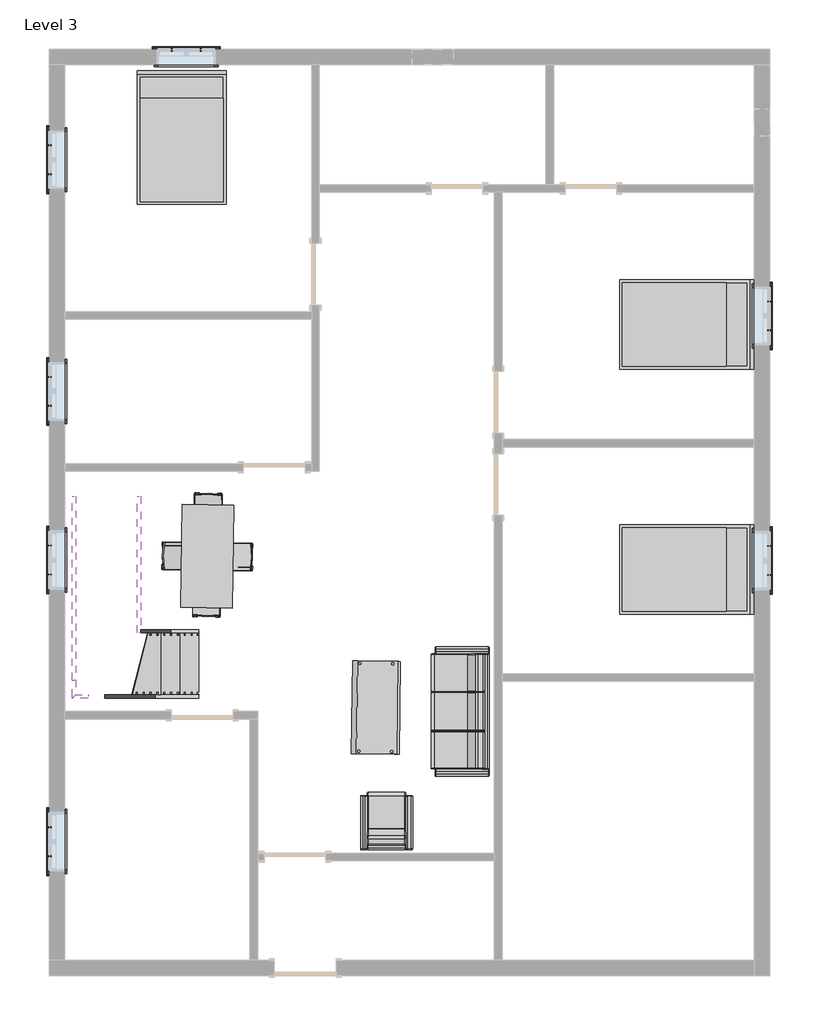
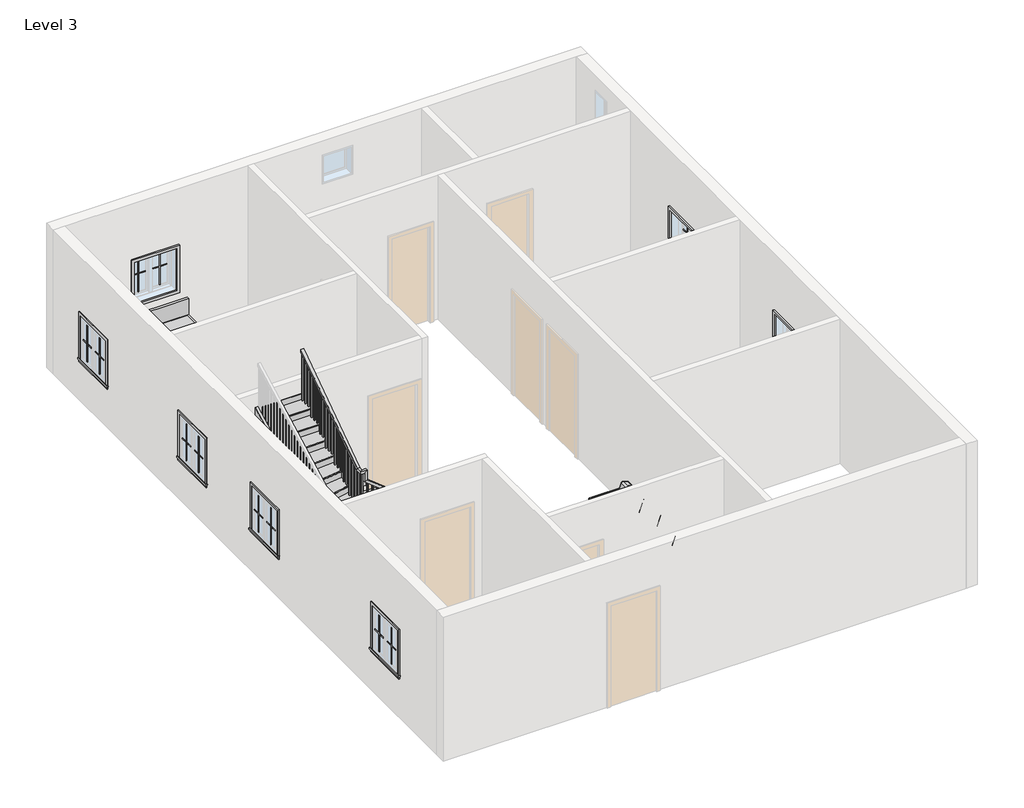
# One storey, part 2 of 2: 29 proxies, 6 furniture elements, 6 members, 1 railing, 1 stair flight.
"""IFC4 building model written with IfcOpenShell, lengths in millimetres."""

from ifc_helpers import new_model, si_unit, frame, origin, place, context, project, spatial, polyline, outline, extrude, faceted_brep, transform, mapped, element, save
from components import modern_coffee_table_17989_modern_coffee_table_17989_d3a860c8, muntin_pattern_2x2_muntin_pattern_2x2_b3fe6957, muntin_pattern_2x2_muntin_pattern_2x2_3e0ecaf2, trim_window_exterior_flat_with_sill_41619996, trim_window_interior_flat_picture_frame_51c85655, furniture_2fc85b74, furniture_29a9adb8, furniture_57072a26, furniture_f28dd14e, furniture_402a1f5e, bed_17739_bed_17739_15c61121, dining_table_w_chairs_11374_0cdfc61b, stair_flight_d75d4b7d

model = new_model("IFC4")

# Units and contexts
model_context = context("Model", 3, world=origin())
ifc_project = project(units=[si_unit("LENGTHUNIT", "METRE", prefix="MILLI")], contexts=[model_context])

# Site, building, storey
site = spatial("IfcSite", under=ifc_project)
building = spatial("IfcBuilding", under=site)
storey = spatial("IfcBuildingStorey", under=building, Name="Level 3", Elevation=3200.4)

# Proxies
placement = place(None, origin())
modern_coffee_table_17989_modern_coffee_table_17989_shape = modern_coffee_table_17989_modern_coffee_table_17989_d3a860c8(model_context)
element("IfcBuildingElementProxy", 1, Name="Modern_Coffee_Table_17989 : Modern_Coffee_Table_17989", ObjectType="Modern_Coffee_Table_17989 : Modern_Coffee_Table_17989", at=placement, inside=storey, context=model_context, shape_type="MappedRepresentation", body=[
    mapped(modern_coffee_table_17989_modern_coffee_table_17989_shape, transform((-2106.8718825, -2116.758017, 3200.4), x_axis=(0.012591066442684793, 0.9999207293810025, 0.0), y_axis=(-0.9999207293810025, 0.012591066442684793, 0.0), z_axis=(0.0, 0.0, 1.0))),
])
muntin_pattern_2x2_muntin_pattern_2x2_shape = muntin_pattern_2x2_muntin_pattern_2x2_b3fe6957(model_context)
element("IfcBuildingElementProxy", 2, Name="Muntin Pattern_2x2 : Muntin Pattern_2x2", ObjectType="Muntin Pattern_2x2 : Muntin Pattern_2x2", at=placement, inside=storey, context=model_context, shape_type="MappedRepresentation", body=[
    mapped(muntin_pattern_2x2_muntin_pattern_2x2_shape, transform((-4775.9474931, 7386.6685985, 4184.65), x_axis=(1.0, 0.0, 0.0), y_axis=(0.0, 1.0, 0.0), z_axis=(0.0, 0.0, 1.0))),
])
element("IfcBuildingElementProxy", 3, Name="Muntin Pattern_2x2 : Muntin Pattern_2x2", ObjectType="Muntin Pattern_2x2 : Muntin Pattern_2x2", at=placement, inside=storey, context=model_context, shape_type="MappedRepresentation", body=[
    mapped(muntin_pattern_2x2_muntin_pattern_2x2_shape, transform((4068.0150069, 3660.8060985, 4184.65), x_axis=(0.0, -1.0, 0.0), y_axis=(1.0, 0.0, 0.0), z_axis=(0.0, 0.0, 1.0))),
])
element("IfcBuildingElementProxy", 4, Name="Muntin Pattern_2x2 : Muntin Pattern_2x2", ObjectType="Muntin Pattern_2x2 : Muntin Pattern_2x2", at=placement, inside=storey, context=model_context, shape_type="MappedRepresentation", body=[
    mapped(muntin_pattern_2x2_muntin_pattern_2x2_shape, transform((4068.0150069, 40.9802908, 4184.65), x_axis=(0.0, -1.0, 0.0), y_axis=(1.0, 0.0, 0.0), z_axis=(0.0, 0.0, 1.0))),
])
element("IfcBuildingElementProxy", 5, Name="Muntin Pattern_2x2 : Muntin Pattern_2x2", ObjectType="Muntin Pattern_2x2 : Muntin Pattern_2x2", at=placement, inside=storey, context=model_context, shape_type="MappedRepresentation", body=[
    mapped(muntin_pattern_2x2_muntin_pattern_2x2_shape, transform((-6580.9349931, 2114.5810985, 4184.65), x_axis=(0.0, 1.0, 0.0), y_axis=(-1.0, 0.0, 0.0), z_axis=(0.0, 0.0, 1.0))),
])
element("IfcBuildingElementProxy", 6, Name="Muntin Pattern_2x2 : Muntin Pattern_2x2", ObjectType="Muntin Pattern_2x2 : Muntin Pattern_2x2", at=placement, inside=storey, context=model_context, shape_type="MappedRepresentation", body=[
    mapped(muntin_pattern_2x2_muntin_pattern_2x2_shape, transform((-6580.9349931, 5543.5810985, 4184.65), x_axis=(0.0, 1.0, 0.0), y_axis=(-1.0, 0.0, 0.0), z_axis=(0.0, 0.0, 1.0))),
])
element("IfcBuildingElementProxy", 7, Name="Muntin Pattern_2x2 : Muntin Pattern_2x2", ObjectType="Muntin Pattern_2x2 : Muntin Pattern_2x2", at=placement, inside=storey, context=model_context, shape_type="MappedRepresentation", body=[
    mapped(muntin_pattern_2x2_muntin_pattern_2x2_shape, transform((-6580.9349931, -4549.7439015, 4184.65), x_axis=(0.0, 1.0, 0.0), y_axis=(-1.0, 0.0, 0.0), z_axis=(0.0, 0.0, 1.0))),
])
element("IfcBuildingElementProxy", 8, Name="Muntin Pattern_2x2 : Muntin Pattern_2x2", ObjectType="Muntin Pattern_2x2 : Muntin Pattern_2x2", at=placement, inside=storey, context=model_context, shape_type="MappedRepresentation", body=[
    mapped(muntin_pattern_2x2_muntin_pattern_2x2_shape, transform((-6580.9349931, -380.9689015, 4184.65), x_axis=(0.0, 1.0, 0.0), y_axis=(-1.0, 0.0, 0.0), z_axis=(0.0, 0.0, 1.0))),
])
muntin_pattern_2x2_muntin_pattern_2x2_2_shape = muntin_pattern_2x2_muntin_pattern_2x2_3e0ecaf2(model_context)
element("IfcBuildingElementProxy", 9, Name="Muntin Pattern_2x2 : Muntin Pattern_2x2", ObjectType="Muntin Pattern_2x2 : Muntin Pattern_2x2", at=placement, inside=storey, context=model_context, shape_type="MappedRepresentation", body=[
    mapped(muntin_pattern_2x2_muntin_pattern_2x2_2_shape, transform((-4347.3224931, 7386.6685985, 4184.65), x_axis=(-1.0, 0.0, 0.0), y_axis=(0.0, -1.0, 0.0), z_axis=(0.0, 0.0, 1.0))),
])
element("IfcBuildingElementProxy", 10, Name="Muntin Pattern_2x2 : Muntin Pattern_2x2", ObjectType="Muntin Pattern_2x2 : Muntin Pattern_2x2", at=placement, inside=storey, context=model_context, shape_type="MappedRepresentation", body=[
    mapped(muntin_pattern_2x2_muntin_pattern_2x2_2_shape, transform((4068.0150069, 3232.1810985, 4184.65), x_axis=(0.0, 1.0, 0.0), y_axis=(-1.0, 0.0, 0.0), z_axis=(0.0, 0.0, 1.0))),
])
element("IfcBuildingElementProxy", 11, Name="Muntin Pattern_2x2 : Muntin Pattern_2x2", ObjectType="Muntin Pattern_2x2 : Muntin Pattern_2x2", at=placement, inside=storey, context=model_context, shape_type="MappedRepresentation", body=[
    mapped(muntin_pattern_2x2_muntin_pattern_2x2_2_shape, transform((4068.0150069, -387.6447092, 4184.65), x_axis=(0.0, 1.0, 0.0), y_axis=(-1.0, 0.0, 0.0), z_axis=(0.0, 0.0, 1.0))),
])
element("IfcBuildingElementProxy", 12, Name="Muntin Pattern_2x2 : Muntin Pattern_2x2", ObjectType="Muntin Pattern_2x2 : Muntin Pattern_2x2", at=placement, inside=storey, context=model_context, shape_type="MappedRepresentation", body=[
    mapped(muntin_pattern_2x2_muntin_pattern_2x2_2_shape, transform((-6580.9349931, 2543.2060985, 4184.65), x_axis=(0.0, -1.0, 0.0), y_axis=(1.0, 0.0, 0.0), z_axis=(0.0, 0.0, 1.0))),
])
element("IfcBuildingElementProxy", 13, Name="Muntin Pattern_2x2 : Muntin Pattern_2x2", ObjectType="Muntin Pattern_2x2 : Muntin Pattern_2x2", at=placement, inside=storey, context=model_context, shape_type="MappedRepresentation", body=[
    mapped(muntin_pattern_2x2_muntin_pattern_2x2_2_shape, transform((-6580.9349931, 5972.2060985, 4184.65), x_axis=(0.0, -1.0, 0.0), y_axis=(1.0, 0.0, 0.0), z_axis=(0.0, 0.0, 1.0))),
])
element("IfcBuildingElementProxy", 14, Name="Muntin Pattern_2x2 : Muntin Pattern_2x2", ObjectType="Muntin Pattern_2x2 : Muntin Pattern_2x2", at=placement, inside=storey, context=model_context, shape_type="MappedRepresentation", body=[
    mapped(muntin_pattern_2x2_muntin_pattern_2x2_2_shape, transform((-6580.9349931, -4121.1189015, 4184.65), x_axis=(0.0, -1.0, 0.0), y_axis=(1.0, 0.0, 0.0), z_axis=(0.0, 0.0, 1.0))),
])
element("IfcBuildingElementProxy", 15, Name="Muntin Pattern_2x2 : Muntin Pattern_2x2", ObjectType="Muntin Pattern_2x2 : Muntin Pattern_2x2", at=placement, inside=storey, context=model_context, shape_type="MappedRepresentation", body=[
    mapped(muntin_pattern_2x2_muntin_pattern_2x2_2_shape, transform((-6580.9349931, 47.6560985, 4184.65), x_axis=(0.0, -1.0, 0.0), y_axis=(1.0, 0.0, 0.0), z_axis=(0.0, 0.0, 1.0))),
])
trim_window_exterior_flat_with_sill_shape = trim_window_exterior_flat_with_sill_41619996(model_context)
element("IfcBuildingElementProxy", 16, Name="Trim-Window-Exterior-Flat : with Sill", ObjectType="Trim-Window-Exterior-Flat : with Sill", at=placement, inside=storey, context=model_context, shape_type="MappedRepresentation", body=[
    mapped(trim_window_exterior_flat_with_sill_shape, transform((-4561.6349931, 7396.1935985, 5029.2), x_axis=(-1.0, 0.0, 0.0), y_axis=(0.0, 0.0, 1.0), z_axis=(0.0, 1.0, 0.0))),
])
element("IfcBuildingElementProxy", 17, Name="Trim-Window-Exterior-Flat : with Sill", ObjectType="Trim-Window-Exterior-Flat : with Sill", at=placement, inside=storey, context=model_context, shape_type="MappedRepresentation", body=[
    mapped(trim_window_exterior_flat_with_sill_shape, transform((4077.5400069, 3446.4935985, 5029.2), x_axis=(0.0, 1.0, 0.0), y_axis=(0.0, 0.0, 1.0), z_axis=(1.0, 0.0, 0.0))),
])
element("IfcBuildingElementProxy", 18, Name="Trim-Window-Exterior-Flat : with Sill", ObjectType="Trim-Window-Exterior-Flat : with Sill", at=placement, inside=storey, context=model_context, shape_type="MappedRepresentation", body=[
    mapped(trim_window_exterior_flat_with_sill_shape, transform((4077.5400069, -173.3322092, 5029.2), x_axis=(0.0, 1.0, 0.0), y_axis=(0.0, 0.0, 1.0), z_axis=(1.0, 0.0, 0.0))),
])
element("IfcBuildingElementProxy", 19, Name="Trim-Window-Exterior-Flat : with Sill", ObjectType="Trim-Window-Exterior-Flat : with Sill", at=placement, inside=storey, context=model_context, shape_type="MappedRepresentation", body=[
    mapped(trim_window_exterior_flat_with_sill_shape, transform((-6590.4599931, 2328.8935985, 5029.2), x_axis=(0.0, -1.0, 0.0), y_axis=(0.0, 0.0, 1.0), z_axis=(-1.0, 0.0, 0.0))),
])
element("IfcBuildingElementProxy", 20, Name="Trim-Window-Exterior-Flat : with Sill", ObjectType="Trim-Window-Exterior-Flat : with Sill", at=placement, inside=storey, context=model_context, shape_type="MappedRepresentation", body=[
    mapped(trim_window_exterior_flat_with_sill_shape, transform((-6590.4599931, 5757.8935985, 5029.2), x_axis=(0.0, -1.0, 0.0), y_axis=(0.0, 0.0, 1.0), z_axis=(-1.0, 0.0, 0.0))),
])
element("IfcBuildingElementProxy", 21, Name="Trim-Window-Exterior-Flat : with Sill", ObjectType="Trim-Window-Exterior-Flat : with Sill", at=placement, inside=storey, context=model_context, shape_type="MappedRepresentation", body=[
    mapped(trim_window_exterior_flat_with_sill_shape, transform((-6590.4599931, -4335.4314015, 5029.2), x_axis=(0.0, -1.0, 0.0), y_axis=(0.0, 0.0, 1.0), z_axis=(-1.0, 0.0, 0.0))),
])
element("IfcBuildingElementProxy", 22, Name="Trim-Window-Exterior-Flat : with Sill", ObjectType="Trim-Window-Exterior-Flat : with Sill", at=placement, inside=storey, context=model_context, shape_type="MappedRepresentation", body=[
    mapped(trim_window_exterior_flat_with_sill_shape, transform((-6590.4599931, -166.6564015, 5029.2), x_axis=(0.0, -1.0, 0.0), y_axis=(0.0, 0.0, 1.0), z_axis=(-1.0, 0.0, 0.0))),
])
trim_window_interior_flat_picture_frame_shape = trim_window_interior_flat_picture_frame_51c85655(model_context)
element("IfcBuildingElementProxy", 23, Name="Trim-Window-Interior-Flat : Picture Frame", ObjectType="Trim-Window-Interior-Flat : Picture Frame", at=placement, inside=storey, context=model_context, shape_type="MappedRepresentation", body=[
    mapped(trim_window_interior_flat_picture_frame_shape, transform((-4561.6349931, 7167.5935985, 5029.2), x_axis=(1.0, 0.0, 0.0), y_axis=(0.0, 0.0, 1.0), z_axis=(0.0, -1.0, 0.0))),
])
element("IfcBuildingElementProxy", 24, Name="Trim-Window-Interior-Flat : Picture Frame", ObjectType="Trim-Window-Interior-Flat : Picture Frame", at=placement, inside=storey, context=model_context, shape_type="MappedRepresentation", body=[
    mapped(trim_window_interior_flat_picture_frame_shape, transform((3848.9400069, 3446.4935985, 5029.2), x_axis=(0.0, -1.0, 0.0), y_axis=(0.0, 0.0, 1.0), z_axis=(-1.0, 0.0, 0.0))),
])
element("IfcBuildingElementProxy", 25, Name="Trim-Window-Interior-Flat : Picture Frame", ObjectType="Trim-Window-Interior-Flat : Picture Frame", at=placement, inside=storey, context=model_context, shape_type="MappedRepresentation", body=[
    mapped(trim_window_interior_flat_picture_frame_shape, transform((3848.9400069, -173.3322092, 5029.2), x_axis=(0.0, -1.0, 0.0), y_axis=(0.0, 0.0, 1.0), z_axis=(-1.0, 0.0, 0.0))),
])
element("IfcBuildingElementProxy", 26, Name="Trim-Window-Interior-Flat : Picture Frame", ObjectType="Trim-Window-Interior-Flat : Picture Frame", at=placement, inside=storey, context=model_context, shape_type="MappedRepresentation", body=[
    mapped(trim_window_interior_flat_picture_frame_shape, transform((-6361.8599931, 2328.8935985, 5029.2), x_axis=(0.0, 1.0, 0.0), y_axis=(0.0, 0.0, 1.0), z_axis=(1.0, 0.0, 0.0))),
])
element("IfcBuildingElementProxy", 27, Name="Trim-Window-Interior-Flat : Picture Frame", ObjectType="Trim-Window-Interior-Flat : Picture Frame", at=placement, inside=storey, context=model_context, shape_type="MappedRepresentation", body=[
    mapped(trim_window_interior_flat_picture_frame_shape, transform((-6361.8599931, 5757.8935985, 5029.2), x_axis=(0.0, 1.0, 0.0), y_axis=(0.0, 0.0, 1.0), z_axis=(1.0, 0.0, 0.0))),
])
element("IfcBuildingElementProxy", 28, Name="Trim-Window-Interior-Flat : Picture Frame", ObjectType="Trim-Window-Interior-Flat : Picture Frame", at=placement, inside=storey, context=model_context, shape_type="MappedRepresentation", body=[
    mapped(trim_window_interior_flat_picture_frame_shape, transform((-6361.8599931, -4335.4314015, 5029.2), x_axis=(0.0, 1.0, 0.0), y_axis=(0.0, 0.0, 1.0), z_axis=(1.0, 0.0, 0.0))),
])
element("IfcBuildingElementProxy", 29, Name="Trim-Window-Interior-Flat : Picture Frame", ObjectType="Trim-Window-Interior-Flat : Picture Frame", at=placement, inside=storey, context=model_context, shape_type="MappedRepresentation", body=[
    mapped(trim_window_interior_flat_picture_frame_shape, transform((-6361.8599931, -166.6564015, 5029.2), x_axis=(0.0, 1.0, 0.0), y_axis=(0.0, 0.0, 1.0), z_axis=(1.0, 0.0, 0.0))),
])

# Furniture
furniture_shape = furniture_2fc85b74(model_context)
furniture_2_shape = furniture_29a9adb8(model_context)
furniture_3_shape = furniture_57072a26(model_context)
element("IfcFurniture", 30, at=placement, inside=storey, context=model_context, shape_type="MappedRepresentation", body=[
    mapped(furniture_shape, transform((-877.7263413, -2408.2064015, 3200.4), x_axis=(0.0, -1.0, 0.0), y_axis=(1.0, 0.0, 0.0), z_axis=(0.0, 0.0, 1.0))),
    mapped(furniture_2_shape, transform((-877.7263413, -2408.2064015, 3200.4), x_axis=(0.0, -1.0, 0.0), y_axis=(1.0, 0.0, 0.0), z_axis=(0.0, 0.0, 1.0))),
    mapped(furniture_3_shape, transform((-877.7263413, -2408.2064015, 3200.4), x_axis=(0.0, -1.0, 0.0), y_axis=(1.0, 0.0, 0.0), z_axis=(0.0, 0.0, 1.0))),
])
furniture_4_shape = furniture_f28dd14e(model_context)
furniture_5_shape = furniture_402a1f5e(model_context)
element("IfcFurniture", 31, at=placement, inside=storey, context=model_context, shape_type="MappedRepresentation", body=[
    mapped(furniture_4_shape, transform((-1595.4975416, -3653.2527501, 3200.4), x_axis=(-1.0, 0.0, 0.0), y_axis=(0.0, -1.0, 0.0), z_axis=(0.0, 0.0, 1.0))),
    mapped(furniture_5_shape, transform((-1595.4975416, -3653.2527501, 3200.4), x_axis=(-1.0, 0.0, 0.0), y_axis=(0.0, -1.0, 0.0), z_axis=(0.0, 0.0, 1.0))),
])
bed_17739_bed_17739_shape = bed_17739_bed_17739_15c61121(model_context)
element("IfcFurniture", 32, ObjectType="Bed_17739 : Bed_17739", at=placement, inside=storey, context=model_context, shape_type="MappedRepresentation", body=[
    mapped(bed_17739_bed_17739_shape, transform((-4628.3099931, 6062.6935985, 3200.4), x_axis=(1.0, 0.0, 0.0), y_axis=(0.0, 1.0, 0.0), z_axis=(0.0, 0.0, 1.0))),
])
element("IfcFurniture", 33, ObjectType="Bed_17739 : Bed_17739", at=placement, inside=storey, context=model_context, shape_type="MappedRepresentation", body=[
    mapped(bed_17739_bed_17739_shape, transform((2820.2400069, 3319.4935985, 3200.4), x_axis=(0.0, -1.0, 0.0), y_axis=(1.0, 0.0, 0.0), z_axis=(0.0, 0.0, 1.0))),
])
element("IfcFurniture", 34, ObjectType="Bed_17739 : Bed_17739", at=placement, inside=storey, context=model_context, shape_type="MappedRepresentation", body=[
    mapped(bed_17739_bed_17739_shape, transform((2820.2400069, -307.008017, 3200.4), x_axis=(0.0, -1.0, 0.0), y_axis=(1.0, 0.0, 0.0), z_axis=(0.0, 0.0, 1.0))),
])
dining_table_w_chairs_11374_shape = dining_table_w_chairs_11374_0cdfc61b(model_context)
element("IfcFurniture", 35, ObjectType="Dining_Table_w_Chairs_11374", at=placement, inside=storey, context=model_context, shape_type="MappedRepresentation", body=[
    mapped(dining_table_w_chairs_11374_shape, transform((-4154.6586335, -131.9172641, 3200.4), x_axis=(0.015873758475140665, 0.9998740039584353, 0.0), y_axis=(-0.9998740039584353, 0.015873758475140665, 0.0), z_axis=(0.0, 0.0, 1.0))),
])

# Members
element("IfcMember", 36, ObjectType="Stringer - 2\" Width", at=placement, inside=storey, context=model_context, shape_type="SweptSolid", body=[
    extrude(outline(polyline([(3790.4562463, -4378.4230036), (4123.2849999, -4378.4230036), (4838.4971411, -6009.0851964), (4505.6683876, -6009.0851964), (3790.4562463, -4378.4230036)])), frame((0.0, -2211.3564015, 0.0), z_axis=(0.0, 1.0, 0.0), x_axis=(0.0, 0.0, 1.0)), (0.0, 0.0, 1.0), 50.8),
])
element("IfcMember", 37, ObjectType="Stringer - 2\" Width", at=placement, inside=storey, context=model_context, shape_type="SweptSolid", body=[
    extrude(outline(polyline([(-6009.0851964, -2160.5564015), (-6009.0851964, -2211.3564015), (-6247.5599931, -2211.3564015), (-6196.7599931, -2160.5564015), (-6009.0851964, -2160.5564015)])), frame((0.0, 0.0, 4505.6683876), z_axis=(0.0, 0.0, 1.0), x_axis=(1.0, 0.0, 0.0)), (0.0, 0.0, 1.0), 332.8287535),
])
element("IfcMember", 38, ObjectType="Stringer - 2\" Width", at=placement, inside=storey, context=model_context, shape_type="SweptSolid", body=[
    extrude(outline(polyline([(-6196.7599931, -2160.5564015), (-6247.5599931, -2211.3564015), (-6247.5599931, -1942.4030584), (-6196.7599931, -1942.4030584), (-6196.7599931, -2160.5564015)])), frame((0.0, 0.0, 4505.6683876), z_axis=(0.0, 0.0, 1.0), x_axis=(1.0, 0.0, 0.0)), (0.0, 0.0, 1.0), 332.8287535),
])
element("IfcMember", 39, ObjectType="Stringer - 2\" Width", at=placement, inside=storey, context=model_context, shape_type="SweptSolid", body=[
    extrude(outline(polyline([(-1942.4030584, 4505.6683876), (-1942.4030584, 4838.4971411), (775.380588, 6254.0189504), (775.380588, 5921.1901969), (-1942.4030584, 4505.6683876)])), frame((-6247.5599931, 0.0, 0.0), z_axis=(1.0, 0.0, 0.0), x_axis=(0.0, 1.0, 0.0)), (0.0, 0.0, 1.0), 50.8),
])
element("IfcMember", 40, ObjectType="Stringer - 2\" Width", at=placement, inside=storey, context=model_context, shape_type="SweptSolid", body=[
    extrude(outline(polyline([(3635.8922729, -4378.4230036), (4043.034734, -4378.4230036), (4798.5690344, -5231.5599931), (4391.4265733, -5231.5599931), (3635.8922729, -4378.4230036)])), frame((0.0, -1246.1564015, 0.0), z_axis=(0.0, 1.0, 0.0), x_axis=(0.0, 0.0, 1.0)), (0.0, 0.0, 1.0), 50.8),
])
element("IfcMember", 41, ObjectType="Stringer - 2\" Width", at=placement, inside=storey, context=model_context, shape_type="SweptSolid", body=[
    extrude(outline(polyline([(-1246.1564015, 4538.1212805), (-1246.1564015, 4910.3296678), (775.380588, 6327.1693854), (775.380588, 5954.9609981), (-1246.1564015, 4538.1212805)])), frame((-5282.3599931, 0.0, 0.0), z_axis=(1.0, 0.0, 0.0), x_axis=(0.0, 1.0, 0.0)), (0.0, 0.0, 1.0), 50.8),
])

# Railing
element("IfcRailing", 42, ObjectType="Handrail - Rectangular", at=placement, inside=storey, context=model_context, shape_type="SolidModel", body=[
    faceted_brep([(-4378.4230036, -1296.9564015, 4961.4666667), (-4378.4230036, -1296.9564015, 4896.5997378), (-4378.4230036, -1246.1564015, 4896.5997378), (-4378.4230036, -1246.1564015, 4961.4666667), (-5206.1599931, -1296.9564015, 5618.7201542), (-5256.9599931, -1296.9564015, 5594.190286), (-5256.9599931, -1246.1564015, 5594.190286), (-5206.1599931, -1246.1564015, 5618.7201542), (-5206.1599931, -1296.9564015, 5825.5172738), (-5256.9599931, -1296.9564015, 5774.7172738), (-5256.9599931, -1246.1564015, 5774.7172738), (-5206.1599931, -1246.1564015, 5825.5172738), (-5333.1599931, -1296.9564015, 5825.5172738), (-5333.1599931, -1296.9564015, 5774.7172738), (-5282.3599931, -1246.1564015, 5774.7172738), (-5282.3599931, -1246.1564015, 5825.5172738), (-5333.1599931, -1169.9564015, 5825.5172738), (-5333.1599931, -1154.1797661, 5774.7172738), (-5282.3599931, -1154.1797661, 5774.7172738), (-5282.3599931, -1169.9564015, 5825.5172738), (-5333.1599931, 775.380588, 7162.8), (-5282.3599931, 775.380588, 7162.8), (-5282.3599931, 775.380588, 7101.1546698), (-5333.1599931, 775.380588, 7101.1546698)], [[[0, 1, 2, 3]], [[1, 0, 4, 5]], [[2, 1, 5, 6]], [[3, 2, 6, 7]], [[0, 3, 7, 4]], [[5, 4, 8, 9]], [[6, 5, 9, 10]], [[7, 6, 10, 11]], [[4, 7, 11, 8]], [[9, 8, 12, 13]], [[10, 9, 13, 14]], [[11, 10, 14, 15]], [[8, 11, 15, 12]], [[13, 12, 16, 17]], [[14, 13, 17, 18]], [[15, 14, 18, 19]], [[12, 15, 19, 16]], [[20, 21, 22, 23]], [[17, 16, 20, 23]], [[18, 17, 23, 22]], [[19, 18, 22, 21]], [[16, 19, 21, 20]]]),
    extrude(outline(polyline([(750.9185985, 7084.3387679), (769.9685985, 7097.4343066), (769.9685985, 6079.0666667), (750.9185985, 6079.0666667), (750.9185985, 7084.3387679)])), frame((-5317.2849931, 0.0, 0.0), z_axis=(1.0, 0.0, 0.0), x_axis=(0.0, 1.0, 0.0)), (0.0, 0.0, 1.0), 19.05),
    extrude(outline(polyline([(649.3185985, 7014.4958945), (668.3685985, 7027.5914333), (668.3685985, 6079.0666667), (649.3185985, 6079.0666667), (649.3185985, 7014.4958945)])), frame((-5317.2849931, 0.0, 0.0), z_axis=(1.0, 0.0, 0.0), x_axis=(0.0, 1.0, 0.0)), (0.0, 0.0, 1.0), 19.05),
    extrude(outline(polyline([(547.7185985, 6944.6530212), (566.7685985, 6957.7485599), (566.7685985, 6079.0666667), (547.7185985, 6079.0666667), (547.7185985, 6944.6530212)])), frame((-5317.2849931, 0.0, 0.0), z_axis=(1.0, 0.0, 0.0), x_axis=(0.0, 1.0, 0.0)), (0.0, 0.0, 1.0), 19.05),
    extrude(outline(polyline([(446.1185985, 6874.8101478), (465.1685985, 6887.9056866), (465.1685985, 5909.7333333), (446.1185985, 5909.7333333), (446.1185985, 6874.8101478)])), frame((-5317.2849931, 0.0, 0.0), z_axis=(1.0, 0.0, 0.0), x_axis=(0.0, 1.0, 0.0)), (0.0, 0.0, 1.0), 19.05),
    extrude(outline(polyline([(344.5185985, 6804.9672745), (363.5685985, 6818.0628132), (363.5685985, 5909.7333333), (344.5185985, 5909.7333333), (344.5185985, 6804.9672745)])), frame((-5317.2849931, 0.0, 0.0), z_axis=(1.0, 0.0, 0.0), x_axis=(0.0, 1.0, 0.0)), (0.0, 0.0, 1.0), 19.05),
    extrude(outline(polyline([(242.9185985, 6735.1244011), (261.9685985, 6748.2199399), (261.9685985, 5909.7333333), (242.9185985, 5909.7333333), (242.9185985, 6735.1244011)])), frame((-5317.2849931, 0.0, 0.0), z_axis=(1.0, 0.0, 0.0), x_axis=(0.0, 1.0, 0.0)), (0.0, 0.0, 1.0), 19.05),
    extrude(outline(polyline([(141.3185985, 6665.2815278), (160.3685985, 6678.3770665), (160.3685985, 5740.4), (141.3185985, 5740.4), (141.3185985, 6665.2815278)])), frame((-5317.2849931, 0.0, 0.0), z_axis=(1.0, 0.0, 0.0), x_axis=(0.0, 1.0, 0.0)), (0.0, 0.0, 1.0), 19.05),
    extrude(outline(polyline([(39.7185985, 6595.4386544), (58.7685985, 6608.5341932), (58.7685985, 5740.4), (39.7185985, 5740.4), (39.7185985, 6595.4386544)])), frame((-5317.2849931, 0.0, 0.0), z_axis=(1.0, 0.0, 0.0), x_axis=(0.0, 1.0, 0.0)), (0.0, 0.0, 1.0), 19.05),
    extrude(outline(polyline([(-61.8814015, 6525.5957811), (-42.8314015, 6538.6913198), (-42.8314015, 5571.0666667), (-61.8814015, 5571.0666667), (-61.8814015, 6525.5957811)])), frame((-5317.2849931, 0.0, 0.0), z_axis=(1.0, 0.0, 0.0), x_axis=(0.0, 1.0, 0.0)), (0.0, 0.0, 1.0), 19.05),
    extrude(outline(polyline([(-163.4814015, 6455.7529077), (-144.4314015, 6468.8484465), (-144.4314015, 5571.0666667), (-163.4814015, 5571.0666667), (-163.4814015, 6455.7529077)])), frame((-5317.2849931, 0.0, 0.0), z_axis=(1.0, 0.0, 0.0), x_axis=(0.0, 1.0, 0.0)), (0.0, 0.0, 1.0), 19.05),
    extrude(outline(polyline([(-265.0814015, 6385.9100344), (-246.0314015, 6399.0055731), (-246.0314015, 5571.0666667), (-265.0814015, 5571.0666667), (-265.0814015, 6385.9100344)])), frame((-5317.2849931, 0.0, 0.0), z_axis=(1.0, 0.0, 0.0), x_axis=(0.0, 1.0, 0.0)), (0.0, 0.0, 1.0), 19.05),
    extrude(outline(polyline([(-366.6814015, 6316.067161), (-347.6314015, 6329.1626998), (-347.6314015, 5401.7333333), (-366.6814015, 5401.7333333), (-366.6814015, 6316.067161)])), frame((-5317.2849931, 0.0, 0.0), z_axis=(1.0, 0.0, 0.0), x_axis=(0.0, 1.0, 0.0)), (0.0, 0.0, 1.0), 19.05),
    extrude(outline(polyline([(-468.2814015, 6246.2242877), (-449.2314015, 6259.3198264), (-449.2314015, 5401.7333333), (-468.2814015, 5401.7333333), (-468.2814015, 6246.2242877)])), frame((-5317.2849931, 0.0, 0.0), z_axis=(1.0, 0.0, 0.0), x_axis=(0.0, 1.0, 0.0)), (0.0, 0.0, 1.0), 19.05),
    extrude(outline(polyline([(-569.8814015, 6176.3814143), (-550.8314015, 6189.4769531), (-550.8314015, 5401.7333333), (-569.8814015, 5401.7333333), (-569.8814015, 6176.3814143)])), frame((-5317.2849931, 0.0, 0.0), z_axis=(1.0, 0.0, 0.0), x_axis=(0.0, 1.0, 0.0)), (0.0, 0.0, 1.0), 19.05),
    extrude(outline(polyline([(-671.4814015, 6106.538541), (-652.4314015, 6119.6340797), (-652.4314015, 5232.4), (-671.4814015, 5232.4), (-671.4814015, 6106.538541)])), frame((-5317.2849931, 0.0, 0.0), z_axis=(1.0, 0.0, 0.0), x_axis=(0.0, 1.0, 0.0)), (0.0, 0.0, 1.0), 19.05),
    extrude(outline(polyline([(-773.0814015, 6036.6956676), (-754.0314015, 6049.7912064), (-754.0314015, 5232.4), (-773.0814015, 5232.4), (-773.0814015, 6036.6956676)])), frame((-5317.2849931, 0.0, 0.0), z_axis=(1.0, 0.0, 0.0), x_axis=(0.0, 1.0, 0.0)), (0.0, 0.0, 1.0), 19.05),
    extrude(outline(polyline([(-874.6814015, 5966.8527943), (-855.6314015, 5979.948333), (-855.6314015, 5063.0666667), (-874.6814015, 5063.0666667), (-874.6814015, 5966.8527943)])), frame((-5317.2849931, 0.0, 0.0), z_axis=(1.0, 0.0, 0.0), x_axis=(0.0, 1.0, 0.0)), (0.0, 0.0, 1.0), 19.05),
    extrude(outline(polyline([(-976.2814015, 5897.0099209), (-957.2314015, 5910.1054597), (-957.2314015, 5063.0666667), (-976.2814015, 5063.0666667), (-976.2814015, 5897.0099209)])), frame((-5317.2849931, 0.0, 0.0), z_axis=(1.0, 0.0, 0.0), x_axis=(0.0, 1.0, 0.0)), (0.0, 0.0, 1.0), 19.05),
    extrude(outline(polyline([(-1077.8814015, 5827.1670476), (-1058.8314015, 5840.2625863), (-1058.8314015, 4893.7333333), (-1077.8814015, 4893.7333333), (-1077.8814015, 5827.1670476)])), frame((-5317.2849931, 0.0, 0.0), z_axis=(1.0, 0.0, 0.0), x_axis=(0.0, 1.0, 0.0)), (0.0, 0.0, 1.0), 19.05),
    extrude(outline(polyline([(-1179.4814015, 5757.3241742), (-1160.4314015, 5770.419713), (-1160.4314015, 4893.7333333), (-1179.4814015, 4893.7333333), (-1179.4814015, 5757.3241742)])), frame((-5317.2849931, 0.0, 0.0), z_axis=(1.0, 0.0, 0.0), x_axis=(0.0, 1.0, 0.0)), (0.0, 0.0, 1.0), 19.05),
    extrude(outline(polyline([(-5283.2980036, -1262.0314015), (-5283.2980036, -1281.0814015), (-5302.3480036, -1281.0814015), (-5302.3480036, -1262.0314015), (-5283.2980036, -1262.0314015)])), frame((0.0, 0.0, 4724.4), z_axis=(0.0, 0.0, 1.0), x_axis=(1.0, 0.0, 0.0)), (0.0, 0.0, 1.0), 1050.3172738),
    extrude(outline(polyline([(5534.4295097, -5181.6980036), (5549.5559074, -5200.7480036), (4555.0666667, -5200.7480036), (4555.0666667, -5181.6980036), (5534.4295097, -5181.6980036)])), frame((0.0, -1281.0814015, 0.0), z_axis=(0.0, 1.0, 0.0), x_axis=(0.0, 0.0, 1.0)), (0.0, 0.0, 1.0), 19.05),
    extrude(outline(polyline([(5453.7553883, -5080.0980036), (5468.8817861, -5099.1480036), (4385.7333333, -5099.1480036), (4385.7333333, -5080.0980036), (5453.7553883, -5080.0980036)])), frame((0.0, -1281.0814015, 0.0), z_axis=(0.0, 1.0, 0.0), x_axis=(0.0, 0.0, 1.0)), (0.0, 0.0, 1.0), 19.05),
    extrude(outline(polyline([(5373.081267, -4978.4980036), (5388.2076647, -4997.5480036), (4385.7333333, -4997.5480036), (4385.7333333, -4978.4980036), (5373.081267, -4978.4980036)])), frame((0.0, -1281.0814015, 0.0), z_axis=(0.0, 1.0, 0.0), x_axis=(0.0, 0.0, 1.0)), (0.0, 0.0, 1.0), 19.05),
    extrude(outline(polyline([(5292.4071456, -4876.8980036), (5307.5335434, -4895.9480036), (4216.4, -4895.9480036), (4216.4, -4876.8980036), (5292.4071456, -4876.8980036)])), frame((0.0, -1281.0814015, 0.0), z_axis=(0.0, 1.0, 0.0), x_axis=(0.0, 0.0, 1.0)), (0.0, 0.0, 1.0), 19.05),
    extrude(outline(polyline([(5211.7330243, -4775.2980036), (5226.859422, -4794.3480036), (4216.4, -4794.3480036), (4216.4, -4775.2980036), (5211.7330243, -4775.2980036)])), frame((0.0, -1281.0814015, 0.0), z_axis=(0.0, 1.0, 0.0), x_axis=(0.0, 0.0, 1.0)), (0.0, 0.0, 1.0), 19.05),
    extrude(outline(polyline([(5131.0589029, -4673.6980036), (5146.1853007, -4692.7480036), (4216.4, -4692.7480036), (4216.4, -4673.6980036), (5131.0589029, -4673.6980036)])), frame((0.0, -1281.0814015, 0.0), z_axis=(0.0, 1.0, 0.0), x_axis=(0.0, 0.0, 1.0)), (0.0, 0.0, 1.0), 19.05),
    extrude(outline(polyline([(5050.3847816, -4572.0980036), (5065.5111793, -4591.1480036), (4047.0666667, -4591.1480036), (4047.0666667, -4572.0980036), (5050.3847816, -4572.0980036)])), frame((0.0, -1281.0814015, 0.0), z_axis=(0.0, 1.0, 0.0), x_axis=(0.0, 0.0, 1.0)), (0.0, 0.0, 1.0), 19.05),
    extrude(outline(polyline([(4969.7106602, -4470.4980036), (4984.837058, -4489.5480036), (4047.0666667, -4489.5480036), (4047.0666667, -4470.4980036), (4969.7106602, -4470.4980036)])), frame((0.0, -1281.0814015, 0.0), z_axis=(0.0, 1.0, 0.0), x_axis=(0.0, 0.0, 1.0)), (0.0, 0.0, 1.0), 19.05),
    extrude(outline(polyline([(-5298.2349931, -1262.0314015), (-5298.2349931, -1281.0814015), (-5317.2849931, -1281.0814015), (-5317.2849931, -1262.0314015), (-5298.2349931, -1262.0314015)])), frame((0.0, 0.0, 4724.4), z_axis=(0.0, 0.0, 1.0), x_axis=(1.0, 0.0, 0.0)), (0.0, 0.0, 1.0), 1050.3172738),
    extrude(outline(polyline([(756.330588, 7088.059131), (775.380588, 7101.1546698), (775.380588, 6079.0666667), (756.330588, 6079.0666667), (756.330588, 7088.059131)])), frame((-5317.2849931, 0.0, 0.0), z_axis=(1.0, 0.0, 0.0), x_axis=(0.0, 1.0, 0.0)), (0.0, 0.0, 1.0), 19.05),
    extrude(outline(polyline([(4896.5997378, -4378.4230036), (4911.7261355, -4397.4730036), (4047.0666667, -4397.4730036), (4047.0666667, -4378.4230036), (4896.5997378, -4378.4230036)])), frame((0.0, -1281.0814015, 0.0), z_axis=(0.0, 1.0, 0.0), x_axis=(0.0, 0.0, 1.0)), (0.0, 0.0, 1.0), 19.05),
])

# Stair flight
stair_flight_shape = stair_flight_d75d4b7d(model_context)
element("IfcStairFlight", 43, ObjectType="2\" Tread 1\" Nosing 1/4\" Riser", at=placement, inside=storey, context=model_context, shape_type="MappedRepresentation", body=[
    mapped(stair_flight_shape, transform((0.0, 0.0, 0.0), x_axis=(1.0, 0.0, 0.0), y_axis=(0.0, 1.0, 0.0), z_axis=(0.0, 0.0, 1.0))),
])

save(model, "model.ifc")

# Revit data of these elements
# Type "Modern_Coffee_Table_17989 : Modern_Coffee_Table_17989"
#   Default Elevation = 0
# Type "Muntin Pattern_2x2 : Muntin Pattern_2x2"
#   Width [instance default] = 4' - 0"
#   Thickness = 0' - 0 1/2"
#   Height [instance default] = 4' - 0"
#   Distance = 0' - 0 3/4"
#   Interior Material [instance default] = none
#   Exterior Material [instance default] = none
#   Default Elevation = 0
# Type "Trim-Window-Exterior-Flat : with Sill"
#   Trim Width = 0' - 2 1/4"
#   Trim Thickness_Picture Frame = 0' - 1 1/4"
#   Trim Thickness_with Sill = 0' - 0 3/4"
#   Sill Thickness = 0' - 1 1/4"
#   Opening Width [instance default] = 2' - 0"
#   Opening Height [instance default] = 3' - 0"
#   Default Elevation = 4' - 0"
#   Sill = yes
#   Picture Frame = no
#   Trim Material [instance default] = none
# Type "Trim-Window-Interior-Flat : Picture Frame"
#   Trim Thickness_Picture Frame = 0' - 1 1/4"
#   Trim Width = 0' - 2 1/4"
#   Trim Thickness_with Sill = 0' - 0 3/4"
#   Sill Thickness = 0' - 1 1/4"
#   Opening Width [instance default] = 2' - 0"
#   Opening Height [instance default] = 3' - 0"
#   Default Elevation = 4' - 0"
#   Sill = no
#   Picture Frame = yes
#   Trim Material [instance default] = none
# Type
#   Width [instance] = 6' - 3.19685"
#   Default Elevation = 0
# Type
#   Width [instance] = 2' - 6.31496"
#   Default Elevation = 0
# Type "Bed_17739 : Bed_17739"
#   Default Elevation = 0
# Type "Dining_Table_w_Chairs_11374"
#   Default Elevation = 0
#   Assembly Code = ""
# Type "Handrail - Rectangular"
#   Assembly Code = "C2010400"
#   built-in parameter 1008612 = 0.0416667 (stored number, unit not read)
#   built-in parameter 1008611 = 0.0416667 (stored number, unit not read)
#   built-in parameter 1008609 = 0.333333 (stored number, unit not read)
#   built-in parameter 1008604 = 0.166667 (stored number, unit not read)
#   built-in parameter 1008603 = 0.166667 (stored number, unit not read)
#   Railing Height = 3' - 0"
#   built-in parameter 1008630 = 2
#   built-in parameter 1008610 = 2
#   built-in parameter 1008618 = Baluster - Square : 3/4"
# Element 1 (IfcBuildingElementProxy, "Modern_Coffee_Table_17989 : Modern_Coffee_Table_17989")
#   Phase Created = New Construction
#   Materials on its faces: "1 Wood", "1 Glass", "1 Metal"
# Elements 2, 3, 4, 5, 6, 7, 8, 9, 10, 11, 12, 13, 14, 15 (IfcBuildingElementProxy, "Muntin Pattern_2x2 : Muntin Pattern_2x2")
#   Width = 0' - 11 5/8"
#   Height = 2' - 6 1/2"
#   Interior Material = Wood - Stained
#   Exterior Material = Clad - White
#   Phase Created = New Construction
#   Materials on its faces: "Clad - White", "Wood - Stained"
# Elements 16, 17, 18, 19, 20, 21, 22 (IfcBuildingElementProxy, "Trim-Window-Exterior-Flat : with Sill")
#   Opening Width = 2' - 10"
#   Opening Height = 3' - 0"
#   Trim Material = Clad - White
#   Phase Created = New Construction
#   Materials on its faces: "Clad - White"
# Elements 23, 24, 25, 26, 27, 28, 29 (IfcBuildingElementProxy, "Trim-Window-Interior-Flat : Picture Frame")
#   Opening Width = 2' - 10"
#   Opening Height = 3' - 0"
#   Trim Material = Wood - Stained
#   Phase Created = New Construction
#   Materials on its faces: "Wood - Stained"
# Element 30 (IfcFurniture)
#   Width = 6' - 3.19685"
#   Phase Created = New Construction
# Element 31 (IfcFurniture)
#   Width = 2' - 6.31496"
#   Phase Created = New Construction
# Elements 32, 33, 34 (IfcFurniture, "Bed_17739 : Bed_17739")
#   Phase Created = New Construction
#   Materials on its faces: "legs", "sheets", "bed frame", "Blanket"
# Element 35 (IfcFurniture, "Dining_Table_w_Chairs_11374")
#   Phase Created = New Construction
# Elements 36, 37, 38, 39, 40, 41 (IfcMember, "Stringer - 2\" Width")
#   Phase Created = New Construction
# Element 42 (IfcRailing, "Handrail - Rectangular")
#   Phase Created = New Construction
# Element 43 (IfcStairFlight, "2\" Tread 1\" Nosing 1/4\" Riser")
#   Phase Created = New Construction
# Materials
#   "1 Wood": class "Glass", colour RGB 81 52 39, transparency 0, Cost = 0
#   "1 Glass": class "Glass", colour RGB 236 240 239, transparency 0.85, Cost = 0
#   "1 Metal": class "Glass", colour RGB 244 244 244, transparency 0, Cost = 0
#   "Clad - White": class "Wood", colour RGB 242 242 238, transparency 0, Cost = 0
#   "Wood - Stained": class "Wood", colour RGB 224 178 126, transparency 0, Cost = 0
#   "legs": colour RGB 90 73 37, transparency 0, Cost = 0
#   "sheets": colour RGB 200 195 176, transparency 0, Cost = 0
#   "bed frame": colour RGB 90 73 37, transparency 0, Cost = 0
#   "Blanket": class "System", colour RGB 59 0 1, transparency 0, Cost = 0
